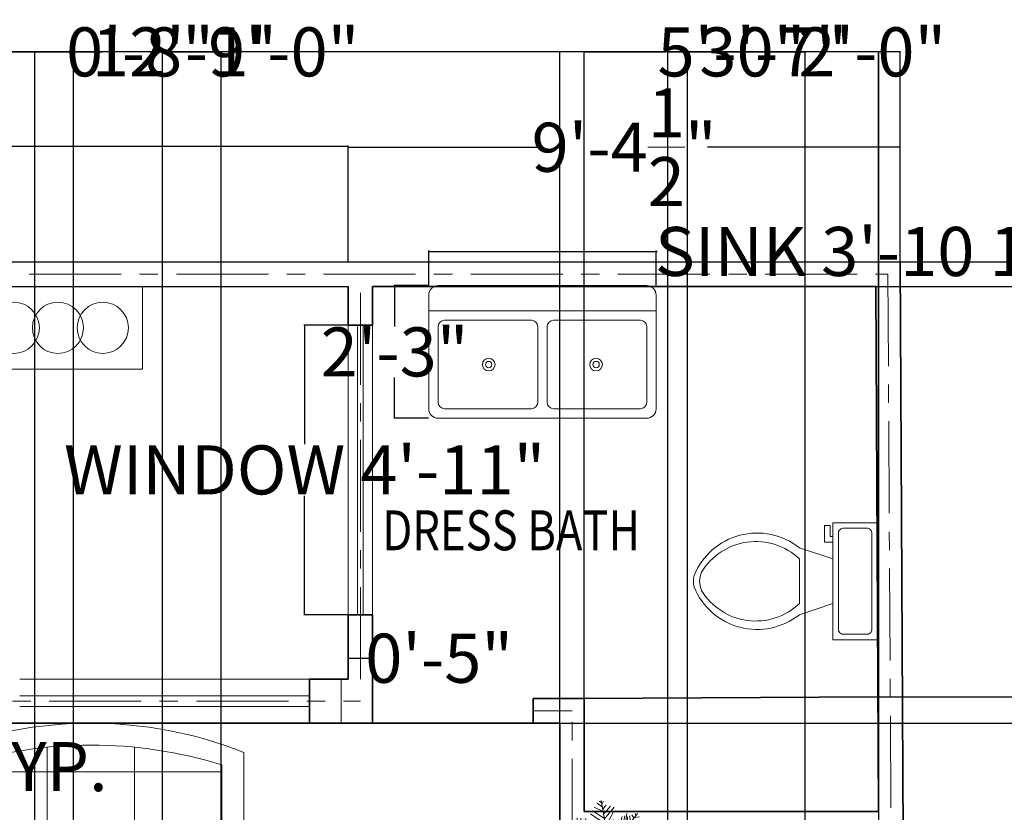
# Model space of a CAD drawing. Units: inches. Extents: x 541 to 1172, y -20 to 887.
# Tile 7 of 8: x 857 to 1058, y 717 to 879. Entities that reach past the tile are written whole.
import ezdxf

# ---------------------------------------------------------------- set-up
doc = ezdxf.new("R2010")
doc.units = ezdxf.units.IN
doc.header["$MEASUREMENT"] = 0
doc.linetypes.add('CENTER', pattern=[50.8, 31.75, -6.35, 6.35, -6.35])
doc.layers.get('0').update_dxf_attribs({"color": 70})
for name, color, linetype, lineweight in [('A-ANNO-DIMS', 2, 'Continuous', 18), ('A-AREA-IDEN', 7, 'Continuous', 20), ('A-FLOR-FIXT', 9, 'Continuous', 18), ('A-FURN', 30, 'Continuous', 18), ('A-WALL-CNTR', 1, 'CENTER', 13), ('C-PROP', 7, 'Continuous', 25), ('L-PLNT', 70, 'Continuous', 18), ('L-SITE-WALL', 7, 'Continuous', 30), ('WALL', 7, 'Continuous', 35), ('WINDOW', 2, 'Continuous', 18)]:
    doc.layers.add(name, color=color, linetype=linetype, lineweight=lineweight)
doc.styles.get("Standard").update_dxf_attribs({"font": 'arial.ttf'})
doc.styles.add('YQ_DIM', font='SUPEROS.SHX', dxfattribs={"width": 0.8, "bigfont": 'HZDX.SHX'})
doc.dimstyles.get("Standard").update_dxf_attribs({"dimtxt": 10, "dimasz": 0.18, "dimexe": 0.18, "dimexo": 0.0625, "dimgap": 0.09, "dimtad": 0, "dimtih": 1, "dimtoh": 1, "dimdec": 1, "dimzin": 0, "dimdsep": 46, "dimlunit": 4, "dimtxsty": 'Standard', "dimcen": 0.09, "dimadec": 0, "dimazin": 0, "dimtfac": 1, "dimtdec": 1, "dimtofl": 0, "dimtmove": 0, "dimatfit": 3, "dimfxl": 1, "dimtolj": 1, "dimtzin": 0, "dimarcsym": 0})

# ---------------------------------------------------------------- blocks, each defined once
blk = doc.blocks.new('*D1')
at = {"layer": 'A-ANNO-DIMS', "color": 0, "lineweight": -2, "transparency": 16777216}
for p, q in [((616.64, 829.74), (616.64, 853.38)), ((616.82, 853.2), (749.39, 853.2)), ((923.96, 853.2), (791.38, 853.2)), ((924.14, 829.74), (924.14, 853.38))]:
    blk.add_line(p, q, dxfattribs=at)
for points in [[(616.82, 853.23), (616.82, 853.17), (616.64, 853.2)], [(923.96, 853.23), (923.96, 853.17), (924.14, 853.2)]]:
    blk.add_solid(points, dxfattribs=at)
at = {"layer": 'Defpoints', "color": 0, "lineweight": -2, "transparency": 16777216}
for p in [(616.64, 853.2), (616.64, 829.68), (924.14, 829.68)]:
    blk.add_point(p, dxfattribs=at)
at = {"layer": 'A-ANNO-DIMS', "color": 0, "transparency": 16777216, "insert": (770.39, 853.2), "char_height": 10, "attachment_point": 5}
blk.add_mtext('\\A1;25\'-7{\\H1x;\\S1/2;}"', dxfattribs=at)
blk = doc.blocks.new('*D2')
at = {"layer": 'A-ANNO-DIMS', "color": 0, "lineweight": -2, "transparency": 16777216}
for p, q in [((924.14, 829.74), (924.14, 853.22)), ((924.32, 853.04), (963.36, 853.04)), ((1036.46, 853.04), (997.41, 853.04)), ((1036.64, 829.74), (1036.64, 853.22))]:
    blk.add_line(p, q, dxfattribs=at)
for points in [[(924.32, 853.07), (924.32, 853.01), (924.14, 853.04)], [(1036.46, 853.07), (1036.46, 853.01), (1036.64, 853.04)]]:
    blk.add_solid(points, dxfattribs=at)
at = {"layer": 'Defpoints', "color": 0, "lineweight": -2, "transparency": 16777216}
for p in [(1036.64, 853.04), (924.14, 829.68), (1036.64, 829.68)]:
    blk.add_point(p, dxfattribs=at)
at = {"layer": 'A-ANNO-DIMS', "color": 0, "transparency": 16777216, "insert": (980.39, 853.04), "char_height": 10, "attachment_point": 5}
blk.add_mtext('\\A1;9\'-4{\\H1x;\\S1/2;}"', dxfattribs=at)
blk = doc.blocks.new('Sofa - Roundback 7 ft.')
for p, q in [((-12.00002, -32.4421), (-12.00003, -6.5971)), ((11.99997, -32.4421), (11.99998, -6.5971)), ((-36.000027, -34), (-36.000027, -11.4696)), ((-35.999844, -13.3819), (35.9998, -13.3819)), ((35.99998, -34), (35.99998, -11.4696)), ((-36.000027, -32.4421), (35.99998, -32.4421))]:
    blk.add_line(p, q)
for points in [[(-36.000027, -34), (-42.000027, -34), (-42.000027, -8)], [(41.99998, -8), (41.99998, -34), (35.99998, -34)]]:
    blk.add_lwpolyline(points)
for centre, radius, start, end in [((0, -114.25), 114.25, 68.43141, 111.5686), ((-0.00001, -127.1968), 121.1968, 72.72033, 107.2797)]:
    blk.add_arc(centre, radius, start, end)
blk = doc.blocks.new('*U7')
for p, q in [((-8.737, 47.138), (-17.069, 52.711)), ((-10.186, 53.64), (-13.084, 55.962)), ((0, 0), (-10.5, 57)), ((-9.099, 51.782), (-6.563, 55.962)), ((-7.65, 43.423), (-2.578, 49.46)), ((-5.839, 35.992), (4.667, 48.067)), ((-3.665, 19.273), (-27.574, 35.527)), ((-5.114, 28.097), (-24.676, 40.636)), ((-7.288, 39.707), (-21.778, 46.673)), ((-5.114, 27.632), (10.463, 46.673)), ((-2.941, 16.486), (8.652, 37.85)), ((22.055, 7.198), (27.489, 32.277)), ((27, 9), (48, 36)), ((27.127, 9.056), (31.112, 35.992)), ((35.096, 32.741), (37.27, 22.524)), ((38.719, 34.134), (41.979, 28.561)), ((44.153, 36.456), (45.239, 32.741)), ((-47.498, 19.737), (-55.83, 18.344)), ((-31.5, 4.5), (-52.5, 25.5)), ((-48.585, 21.131), (-49.309, 29.026)), ((-43.513, 28.561), (-42.427, 15.558)), ((-38.442, 26.239), (-34.819, 7.663)), ((-35.544, 28.097), (-24.314, 3.947)), ((-14.533, 2.09), (-30.834, 25.31)), ((-24.314, 23.917), (-2.941, 13.7)), ((-1.129, 6.734), (9.014, 26.704)), ((3.942, 1.625), (11.187, 24.381)), ((10.101, 3.483), (17.708, 26.239)), ((16.259, 5.805), (23.142, 31.348)), ((31.836, 30.883), (32.561, 16.486)), ((33.285, 16.486), (48.862, 10.913)), ((36.183, 19.737), (48.137, 17.88)), ((40.53, 25.775), (48.862, 24.846)), ((43.791, 29.954), (51.036, 30.883)), ((-40.615, 13.7), (-55.105, 10.913)), ((-33.37, 6.269), (-52.207, 5.34)), ((-28.299, 3.483), (-47.86, -5.805)), ((-21.416, 3.018), (-38.079, -8.128)), ((0, 0), (-31.5, 4.5)), ((-15.982, 2.09), (-30.11, -9.521)), ((0, 0), (-22.5, -19.5)), ((-6.563, 1.161), (-21.416, -8.128)), ((-20.691, 13.7), (-1.129, 4.876)), ((0, 0), (27, 9)), ((0, 0), (18, -22.5)), ((6.478, 1.625), (26.04, -8.592)), ((11.187, 3.483), (30.749, -5.805)), ((18.07, 5.805), (35.096, -3.483)), ((24.229, 7.663), (46.688, 1.625)), ((29.662, 12.307), (48.137, 6.269)), ((-17.431, -15.094), (-42.789, -18.809)), ((-15.257, -12.772), (-30.11, -12.772)), ((-6.563, -5.805), (-19.967, -9.985)), ((-17.069, -15.094), (-12.721, -40.172)), ((-13.446, -11.378), (-8.737, -32.741)), ((-9.461, -8.592), (-6.201, -23.453)), ((-4.752, -3.483), (-3.665, -14.629)), ((2.493, -3.019), (-1.491, -20.202)), ((1.769, -2.555), (24.229, -9.521)), ((5.029, -6.27), (2.131, -25.775)), ((9.014, -11.378), (3.58, -35.992)), ((7.565, -9.056), (32.198, -14.629)), ((12.274, -15.094), (36.907, -18.809)), ((-28.299, -29.026), (-42.789, -31.348)), ((-24.314, -21.596), (-42.427, -22.06)), ((-26.849, -26.24), (-40.253, -25.775)), ((-22.5, -19.5), (-37.5, -45)), ((-29.023, -30.884), (-27.936, -43.887)), ((-25.038, -23.918), (-22.865, -45.281)), ((-20.691, -18.345), (-17.793, -44.352)), ((14.085, -16.951), (6.478, -40.172)), ((18.07, -22.524), (8.289, -45.745)), ((20.244, -30.419), (15.897, -44.816)), ((16.259, -19.738), (36.183, -22.989)), ((18, -22.5), (27, -52.5)), ((18.433, -22.524), (40.53, -29.026)), ((19.157, -25.311), (38.719, -33.206)), ((-30.834, -34.135), (-42.427, -35.528)), ((-34.457, -39.708), (-40.978, -42.494)), ((-32.646, -36.921), (-31.921, -44.352)), ((22.78, -37.85), (19.519, -48.532)), ((21.331, -32.741), (39.081, -40.636)), ((22.78, -38.314), (34.372, -44.816)), ((24.591, -45.745), (23.142, -50.854)), ((24.591, -43.423), (30.749, -47.603)), ((26.764, -49.925), (28.213, -50.854))]:
    blk.add_line(p, q)
blk = doc.blocks.new('WD_WIN4')
at = {"lineweight": -2}
for p, q in [((-0.5, 0.5), (0.5, 0.5)), ((-0.5, 0.12), (0.5, 0.12)), ((-0.5, -0.12), (0.5, -0.12)), ((-0.5, -0.5), (0.5, -0.5))]:
    blk.add_line(p, q, dxfattribs=at)
blk = doc.blocks.new('*U28')
for p, q in [((9.5, -6), (9.5, -2)), ((-10, -8.5), (-8, -8.5)), ((-10, -9.5), (-10, -8.5)), ((-8, -8.5), (-8, -8)), ((-7, -8), (-7, -9.5)), ((-4, -8), (-6, -14)), ((4, -8), (6, -14)), ((-7, -9.5), (-10, -9.5)), ((4, -14), (-4, -14))]:
    blk.add_line(p, q)
blk.add_lwpolyline([(10.5, -8), (10.5, 0), (-10.5, 0), (-10.5, -8)], close=True)
for points in [[(8.5, -1), (-8.5, -1)], [(-9.5, -2), (-9.5, -6)], [(-8.5, -7), (8.5, -7)]]:
    blk.add_lwpolyline(points)
for centre, radius, start, end in [((-8.62, -1.88), 0.884, 81.8699, 188.1301), ((8.62, -1.88), 0.884, 351.8699, 98.1301), ((-8.62, -6.12), 0.884, 171.8699, 278.1301), ((8.62, -6.12), 0.884, 261.8699, 8.1301), ((3.52, -21.58), 12.17, 141.4691, 247.9714), ((4.2, -21.82), 11.33, 136.3677, 238.9468), ((-3.52, -21.58), 12.17, 292.0284, 38.5307), ((-4.2, -21.82), 11.33, 301.053, 43.6321), ((0, -27.88), 4, 245.7318, 294.2682), ((0, -29), 4, 254.8605, 285.1395)]:
    blk.add_arc(centre, radius, start, end)
blk = doc.blocks.new('Sink-double - 36 in top')
for p, q in [((-18, -4), (18, -4)), ((-0.75, -18.5), (-0.75, -6.5)), ((0.75, -6.5), (0.75, -18.5))]:
    blk.add_line(p, q)
for points in [[(-16.5, 0), (16.5, 0)], [(-18, -19.5), (-18, -1.5)], [(18, -1.5), (18, -19.5)], [(-15.5, -5.5), (-1.75, -5.5)], [(1.75, -5.5), (15.5, -5.5)], [(-16.5, -18.5), (-16.5, -6.5)], [(16.5, -6.5), (16.5, -18.5)], [(-1.75, -19.5), (-15.5, -19.5)], [(15.5, -19.5), (1.75, -19.5)], [(16.5, -21), (-16.5, -21)]]:
    blk.add_lwpolyline(points)
for centre, radius in [((-8.5, -12.5), 1), ((-8.5, -12.5), 0.5), ((8.5, -12.5), 1), ((8.5, -12.5), 0.5)]:
    blk.add_circle(centre, radius)
for centre, radius, start, end in [((-16.5, -1.5), 1.5, 90, 180), ((16.5, -1.5), 1.5, 0, 90), ((-15.5, -6.5), 1, 90, 180), ((-1.75, -6.5), 1, 0, 90), ((1.75, -6.5), 1, 90, 180), ((15.5, -6.5), 1, 0, 90), ((-15.5, -18.5), 1, 180, 270), ((-1.75, -18.5), 1, 270, 0), ((1.75, -18.5), 1, 180, 270), ((15.5, -18.5), 1, 270, 0), ((-16.5, -19.5), 1.5, 180, 270), ((16.5, -19.5), 1.5, 270, 0)]:
    blk.add_arc(centre, radius, start, end)
blk = doc.blocks.new('PLANTER-THREE-ROUND')
blk.add_lwpolyline([(34.49, 16.89), (0, 16.89), (0, 0), (34.49, 0)], close=True)
for centre in [(8.25, 8.45), (17.25, 8.45), (26.39, 8.45)]:
    blk.add_circle(centre, 5.21)
blk = doc.blocks.new('*D39')
at = {"layer": 'A-ANNO-DIMS', "color": 0, "lineweight": -2, "transparency": 16777216}
for p, q in [((684.16, 735.59), (684.16, 726.62)), ((743.21, 735.59), (743.21, 726.62)), ((684.34, 726.8), (743.03, 726.8)), ((743.21, 726.8), (743.39, 726.8))]:
    blk.add_line(p, q, dxfattribs=at)
for points in [[(684.34, 726.83), (684.34, 726.77), (684.16, 726.8)], [(743.03, 726.83), (743.03, 726.77), (743.21, 726.8)]]:
    blk.add_solid(points, dxfattribs=at)
at = {"layer": 'Defpoints', "color": 0, "lineweight": -2, "transparency": 16777216}
for p in [(684.16, 735.65), (743.21, 735.65), (743.21, 726.8)]:
    blk.add_point(p, dxfattribs=at)
at = {"layer": 'A-ANNO-DIMS', "color": 0, "transparency": 16777216, "insert": (810.64, 726.8), "char_height": 10, "attachment_point": 5}
blk.add_mtext('\\A1;WINDOW 4\'-11" TYP.', dxfattribs=at)
blk = doc.blocks.new('*D41')
at = {"layer": 'A-ANNO-DIMS', "color": 0, "lineweight": -2, "transparency": 16777216}
for p, q in [((924.07, 816.81), (915.1, 816.81)), ((915.28, 816.63), (915.28, 792.54)), ((915.28, 757.93), (915.28, 782.01)), ((924.07, 757.75), (915.1, 757.75))]:
    blk.add_line(p, q, dxfattribs=at)
for points in [[(915.25, 816.63), (915.31, 816.63), (915.28, 816.81)], [(915.25, 757.93), (915.31, 757.93), (915.28, 757.75)]]:
    blk.add_solid(points, dxfattribs=at)
at = {"layer": 'Defpoints', "color": 0, "lineweight": -2, "transparency": 16777216}
for p in [(924.14, 816.81), (915.28, 757.75), (924.14, 757.75)]:
    blk.add_point(p, dxfattribs=at)
at = {"layer": 'A-ANNO-DIMS', "color": 0, "transparency": 16777216, "insert": (915.28, 787.28), "char_height": 10, "attachment_point": 5}
blk.add_mtext('\\A1;WINDOW 4\'-11"', dxfattribs=at)
blk = doc.blocks.new('*D42')
at = {"layer": 'A-ANNO-DIMS', "color": 0, "lineweight": -2, "transparency": 16777216}
for p, q in [((924.14, 757.69), (924.14, 748.71)), ((929.14, 757.69), (929.14, 748.71)), ((924.32, 748.89), (928.96, 748.89)), ((929.14, 748.89), (929.32, 748.89))]:
    blk.add_line(p, q, dxfattribs=at)
for points in [[(924.32, 748.92), (924.32, 748.86), (924.14, 748.89)], [(928.96, 748.92), (928.96, 748.86), (929.14, 748.89)]]:
    blk.add_solid(points, dxfattribs=at)
at = {"layer": 'Defpoints', "color": 0, "lineweight": -2, "transparency": 16777216}
for p in [(924.14, 757.75), (929.14, 757.75), (929.14, 748.89)]:
    blk.add_point(p, dxfattribs=at)
at = {"layer": 'A-ANNO-DIMS', "color": 0, "transparency": 16777216, "insert": (942.7, 748.89), "char_height": 10, "attachment_point": 5}
blk.add_mtext('\\A1;0\'-5"', dxfattribs=at)
blk = doc.blocks.new('*D53')
at = {"layer": 'A-ANNO-DIMS', "color": 0, "lineweight": -2, "transparency": 16777216}
for p, q in [((940.56, 824.91), (940.56, 831.98)), ((940.74, 831.8), (986.74, 831.8)), ((986.92, 824.91), (986.92, 831.98)), ((986.92, 831.8), (987.1, 831.8))]:
    blk.add_line(p, q, dxfattribs=at)
for points in [[(940.74, 831.83), (940.74, 831.77), (940.56, 831.8)], [(986.74, 831.83), (986.74, 831.77), (986.92, 831.8)]]:
    blk.add_solid(points, dxfattribs=at)
at = {"layer": 'Defpoints', "color": 0, "lineweight": -2, "transparency": 16777216}
for p in [(986.92, 831.8), (940.56, 824.85), (986.92, 824.85)]:
    blk.add_point(p, dxfattribs=at)
at = {"layer": 'A-ANNO-DIMS', "color": 0, "transparency": 16777216, "insert": (1034.24, 831.8), "char_height": 10, "attachment_point": 5}
blk.add_mtext('\\A1;SINK 3\'-10 1/2"', dxfattribs=at)
blk = doc.blocks.new('*D54')
at = {"layer": 'A-ANNO-DIMS', "color": 0, "lineweight": -2, "transparency": 16777216}
for p, q in [((940.5, 824.85), (933.43, 824.85)), ((933.61, 824.67), (933.61, 816.53)), ((933.61, 797.99), (933.61, 806.13)), ((940.5, 797.81), (933.43, 797.81))]:
    blk.add_line(p, q, dxfattribs=at)
for points in [[(933.58, 824.67), (933.64, 824.67), (933.61, 824.85)], [(933.58, 797.99), (933.64, 797.99), (933.61, 797.81)]]:
    blk.add_solid(points, dxfattribs=at)
at = {"layer": 'Defpoints', "color": 0, "lineweight": -2, "transparency": 16777216}
for p in [(933.61, 824.85), (940.56, 824.85), (940.56, 797.81)]:
    blk.add_point(p, dxfattribs=at)
at = {"layer": 'A-ANNO-DIMS', "color": 0, "transparency": 16777216, "insert": (933.61, 811.33), "char_height": 10, "attachment_point": 5}
blk.add_mtext('\\A1;2\'-3"', dxfattribs=at)
blk = doc.blocks.new('*D69')
at = {"layer": 'A-ANNO-DIMS', "color": 0, "lineweight": -2, "transparency": 16777216}
for p, q in [((616.64, 829.74), (616.64, 872.66)), ((616.82, 872.48), (809.37, 872.48)), ((1036.46, 872.48), (843.9, 872.48)), ((1036.64, 829.74), (1036.64, 872.66))]:
    blk.add_line(p, q, dxfattribs=at)
for points in [[(616.82, 872.51), (616.82, 872.45), (616.64, 872.48)], [(1036.46, 872.51), (1036.46, 872.45), (1036.64, 872.48)]]:
    blk.add_solid(points, dxfattribs=at)
at = {"layer": 'Defpoints', "color": 0, "lineweight": -2, "transparency": 16777216}
for p in [(1036.64, 872.48), (616.64, 829.68), (1036.64, 829.68)]:
    blk.add_point(p, dxfattribs=at)
at = {"layer": 'A-ANNO-DIMS', "color": 0, "transparency": 16777216, "insert": (826.64, 872.48), "char_height": 10, "attachment_point": 5}
blk.add_mtext('\\A1;35\'-0"', dxfattribs=at)
blk = doc.blocks.new('*D70')
at = {"layer": 'A-ANNO-DIMS', "color": 0, "lineweight": -2, "transparency": 16777216}
for p, q in [((1036.7, 829.68), (1143.21, 829.68)), ((1143.03, 829.5), (1143.03, 444.36)), ((1143.03, 48.83), (1143.03, 433.97)), ((1037.35, 48.65), (1143.21, 48.65))]:
    blk.add_line(p, q, dxfattribs=at)
for points in [[(1143, 829.5), (1143.06, 829.5), (1143.03, 829.68)], [(1143, 48.83), (1143.06, 48.83), (1143.03, 48.65)]]:
    blk.add_solid(points, dxfattribs=at)
at = {"layer": 'Defpoints', "color": 0, "lineweight": -2, "transparency": 16777216}
for p in [(1036.64, 829.68), (1037.28, 48.65), (1143.03, 48.65)]:
    blk.add_point(p, dxfattribs=at)
at = {"layer": 'A-ANNO-DIMS', "color": 0, "transparency": 16777216, "insert": (1143.03, 439.17), "char_height": 10, "attachment_point": 5}
blk.add_mtext('\\A1;65\'-1"', dxfattribs=at)
blk = doc.blocks.new('*D76')
at = {"layer": 'A-ANNO-DIMS', "color": 0, "lineweight": -2, "transparency": 16777216}
for p, q in [((814.28, 735.72), (814.28, 872.66)), ((814.46, 872.48), (873.99, 872.48)), ((967.1, 872.48), (907.58, 872.48)), ((967.28, 735.72), (967.28, 872.66))]:
    blk.add_line(p, q, dxfattribs=at)
for points in [[(814.46, 872.51), (814.46, 872.45), (814.28, 872.48)], [(967.1, 872.51), (967.1, 872.45), (967.28, 872.48)]]:
    blk.add_solid(points, dxfattribs=at)
at = {"layer": 'Defpoints', "color": 0, "lineweight": -2, "transparency": 16777216}
for p in [(967.28, 872.48), (814.28, 735.65), (967.28, 735.65)]:
    blk.add_point(p, dxfattribs=at)
at = {"layer": 'A-ANNO-DIMS', "color": 0, "transparency": 16777216, "insert": (890.78, 872.48), "char_height": 10, "attachment_point": 5}
blk.add_mtext('\\A1;12\'-9"', dxfattribs=at)
blk = doc.blocks.new('*D77')
at = {"layer": 'A-ANNO-DIMS', "color": 0, "lineweight": -2, "transparency": 16777216}
for p, q in [((972.28, 717.72), (972.28, 872.66)), ((972.46, 872.48), (988.89, 872.48)), ((1032.08, 872.48), (1015.65, 872.48)), ((1032.26, 717.72), (1032.26, 872.66))]:
    blk.add_line(p, q, dxfattribs=at)
for points in [[(972.46, 872.51), (972.46, 872.45), (972.28, 872.48)], [(1032.08, 872.51), (1032.08, 872.45), (1032.26, 872.48)]]:
    blk.add_solid(points, dxfattribs=at)
at = {"layer": 'Defpoints', "color": 0, "lineweight": -2, "transparency": 16777216}
for p in [(1032.26, 872.48), (972.28, 717.65), (1032.26, 717.65)]:
    blk.add_point(p, dxfattribs=at)
at = {"layer": 'A-ANNO-DIMS', "color": 0, "transparency": 16777216, "insert": (1002.27, 872.48), "char_height": 10, "attachment_point": 5}
blk.add_mtext('\\A1;5\'-0"', dxfattribs=at)
blk = doc.blocks.new('*D79')
at = {"layer": 'A-ANNO-DIMS', "color": 0, "lineweight": -2, "transparency": 16777216}
for p, q in [((1031.73, 824.68), (1143.21, 824.68)), ((1143.03, 824.5), (1143.03, 788.09)), ((1143.03, 741.17), (1143.03, 777.57)), ((1032.19, 740.99), (1143.21, 740.99))]:
    blk.add_line(p, q, dxfattribs=at)
for points in [[(1143, 824.5), (1143.06, 824.5), (1143.03, 824.68)], [(1143, 741.17), (1143.06, 741.17), (1143.03, 740.99)]]:
    blk.add_solid(points, dxfattribs=at)
at = {"layer": 'Defpoints', "color": 0, "lineweight": -2, "transparency": 16777216}
for p in [(1031.66, 824.68), (1032.13, 740.99), (1143.03, 740.99)]:
    blk.add_point(p, dxfattribs=at)
at = {"layer": 'A-ANNO-DIMS', "color": 0, "transparency": 16777216, "insert": (1143.03, 782.83), "char_height": 10, "attachment_point": 5}
blk.add_mtext('\\A1;6\'-11 1/2"', dxfattribs=at)
blk = doc.blocks.new('*D89')
at = {"layer": 'A-ANNO-DIMS', "color": 0, "lineweight": -2, "transparency": 16777216}
for p, q in [((989.28, 430.72), (989.28, 872.66)), ((989.46, 872.48), (997.41, 872.48)), ((1032.1, 872.48), (1024.16, 872.48)), ((1032.28, 430.72), (1032.28, 872.66))]:
    blk.add_line(p, q, dxfattribs=at)
for points in [[(989.46, 872.51), (989.46, 872.45), (989.28, 872.48)], [(1032.1, 872.51), (1032.1, 872.45), (1032.28, 872.48)]]:
    blk.add_solid(points, dxfattribs=at)
at = {"layer": 'Defpoints', "color": 0, "lineweight": -2, "transparency": 16777216}
for p in [(1032.28, 872.48), (989.28, 430.65), (1032.28, 430.65)]:
    blk.add_point(p, dxfattribs=at)
at = {"layer": 'A-ANNO-DIMS', "color": 0, "transparency": 16777216, "insert": (1010.78, 872.48), "char_height": 10, "attachment_point": 5}
blk.add_mtext('\\A1;3\'-7"', dxfattribs=at)
blk = doc.blocks.new('*D97')
at = {"layer": 'A-ANNO-DIMS', "color": 0, "lineweight": -2, "transparency": 16777216}
for p, q in [((886.28, 430.72), (886.28, 872.66)), ((886.46, 872.48), (898.1, 872.48)), ((898.28, 430.72), (898.28, 872.66)), ((898.28, 872.48), (898.46, 872.48))]:
    blk.add_line(p, q, dxfattribs=at)
for points in [[(886.46, 872.51), (886.46, 872.45), (886.28, 872.48)], [(898.1, 872.51), (898.1, 872.45), (898.28, 872.48)]]:
    blk.add_solid(points, dxfattribs=at)
at = {"layer": 'Defpoints', "color": 0, "lineweight": -2, "transparency": 16777216}
for p in [(898.28, 872.48), (886.28, 430.65), (898.28, 430.65)]:
    blk.add_point(p, dxfattribs=at)
at = {"layer": 'A-ANNO-DIMS', "color": 0, "transparency": 16777216, "insert": (911.37, 872.48), "char_height": 10, "attachment_point": 5}
blk.add_mtext('\\A1;1\'-0"', dxfattribs=at)
blk = doc.blocks.new('*D98')
at = {"layer": 'A-ANNO-DIMS', "color": 0, "lineweight": -2, "transparency": 16777216}
for p, q in [((993.28, 326.72), (993.28, 872.66)), ((993.46, 872.48), (1017.14, 872.48)), ((1017.32, 326.72), (1017.32, 872.66)), ((1017.32, 872.48), (1017.5, 872.48))]:
    blk.add_line(p, q, dxfattribs=at)
for points in [[(993.46, 872.51), (993.46, 872.45), (993.28, 872.48)], [(1017.14, 872.51), (1017.14, 872.45), (1017.32, 872.48)]]:
    blk.add_solid(points, dxfattribs=at)
at = {"layer": 'Defpoints', "color": 0, "lineweight": -2, "transparency": 16777216}
for p in [(1017.32, 872.48), (993.28, 326.65), (1017.32, 326.65)]:
    blk.add_point(p, dxfattribs=at)
at = {"layer": 'A-ANNO-DIMS', "color": 0, "transparency": 16777216, "insert": (1030.97, 872.48), "char_height": 10, "attachment_point": 5}
blk.add_mtext('\\A1;2\'-0"', dxfattribs=at)
blk = doc.blocks.new('*D101')
at = {"layer": 'A-ANNO-DIMS', "color": 0, "lineweight": -2, "transparency": 16777216}
for p, q in [((805.35, 735.65), (1143.21, 735.65)), ((1143.03, 735.47), (1143.03, 730.35)), ((1143.03, 714.83), (1143.03, 719.96)), ((805.35, 714.65), (1143.21, 714.65))]:
    blk.add_line(p, q, dxfattribs=at)
for points in [[(1143, 735.47), (1143.06, 735.47), (1143.03, 735.65)], [(1143, 714.83), (1143.06, 714.83), (1143.03, 714.65)]]:
    blk.add_solid(points, dxfattribs=at)
at = {"layer": 'Defpoints', "color": 0, "lineweight": -2, "transparency": 16777216}
for p in [(805.28, 735.65), (1143.03, 735.65), (805.28, 714.65)]:
    blk.add_point(p, dxfattribs=at)
at = {"layer": 'A-ANNO-DIMS', "color": 0, "transparency": 16777216, "insert": (1143.03, 725.15), "char_height": 10, "attachment_point": 5}
blk.add_mtext('\\A1;1\'-9"', dxfattribs=at)
blk = doc.blocks.new('*D104')
at = {"layer": 'A-ANNO-DIMS', "color": 0, "lineweight": -2, "transparency": 16777216}
for p, q in [((860.28, 177.72), (860.28, 872.66)), ((860.46, 872.48), (867.98, 872.48)), ((868.16, 177.72), (868.16, 872.66)), ((868.16, 872.48), (868.34, 872.48))]:
    blk.add_line(p, q, dxfattribs=at)
for points in [[(860.46, 872.51), (860.46, 872.45), (860.28, 872.48)], [(867.98, 872.51), (867.98, 872.45), (868.16, 872.48)]]:
    blk.add_solid(points, dxfattribs=at)
at = {"layer": 'Defpoints', "color": 0, "lineweight": -2, "transparency": 16777216}
for p in [(868.16, 872.48), (860.28, 177.65), (868.16, 177.65)]:
    blk.add_point(p, dxfattribs=at)
at = {"layer": 'A-ANNO-DIMS', "color": 0, "transparency": 16777216, "insert": (881.72, 872.48), "char_height": 10, "attachment_point": 5}
blk.add_mtext('\\A1;0\'-8"', dxfattribs=at)
blk = doc.blocks.new('*D107')
at = {"layer": 'A-ANNO-DIMS', "color": 0, "lineweight": -2, "transparency": 16777216}
for p, q in [((967.22, 735.65), (573.66, 735.65)), ((573.84, 735.47), (573.84, 668.85)), ((573.84, 591.83), (573.84, 658.46)), ((967.22, 591.65), (573.66, 591.65))]:
    blk.add_line(p, q, dxfattribs=at)
for points in [[(573.81, 735.47), (573.87, 735.47), (573.84, 735.65)], [(573.81, 591.83), (573.87, 591.83), (573.84, 591.65)]]:
    blk.add_solid(points, dxfattribs=at)
at = {"layer": 'Defpoints', "color": 0, "lineweight": -2, "transparency": 16777216}
for p in [(967.28, 735.65), (573.84, 591.65), (967.28, 591.65)]:
    blk.add_point(p, dxfattribs=at)
at = {"layer": 'A-ANNO-DIMS', "color": 0, "transparency": 16777216, "insert": (573.84, 663.65), "char_height": 10, "attachment_point": 5}
blk.add_mtext('\\A1;12\'-0"', dxfattribs=at)

msp = doc.modelspace()

# ---------------------------------------------------------------- linework, layer by layer
at = {"layer": 'A-WALL-CNTR', "ltscale": 0.590551}
for p, q in [((619.14, 827.18), (1034.15, 827.18)), ((1034.15, 827.18), (1034.77, 715.15)), ((926.64, 744.65), (926.64, 824.68)), ((922.7, 735.65), (922.7, 744.65)), ((743.21, 740.15), (926.64, 740.15)), ((961.84, 738.15), (969.78, 738.15)), ((969.78, 589.65), (969.78, 738.15))]:
    msp.add_line(p, q, dxfattribs=at)
at = {"layer": 'C-PROP'}
msp.add_line((616.64, 829.68), (1036.64, 829.68), dxfattribs=at)
at = {"layer": 'L-SITE-WALL'}
for p, q in [((616.64, 829.68), (1036.64, 829.68)), ((621.64, 824.68), (924.14, 824.68))]:
    msp.add_line(p, q, dxfattribs=at)
at = {"layer": 'WALL'}
for p, q in [((1036.64, 829.68), (1037.28, 712.65)), ((924.14, 816.81), (924.14, 824.68)), ((929.14, 824.68), (1031.66, 824.68)), ((929.14, 816.81), (929.14, 824.68)), ((1031.66, 824.68), (1032.26, 717.65)), ((924.14, 816.81), (929.14, 816.81)), ((924.14, 744.65), (924.14, 757.75)), ((924.14, 757.75), (929.14, 757.75)), ((929.14, 735.65), (929.14, 757.75)), ((916.26, 744.65), (924.14, 744.65)), ((916.26, 744.65), (916.26, 735.65)), ((972.28, 740.65), (961.84, 740.65)), ((961.84, 740.65), (961.84, 735.65)), ((972.28, 740.65), (1032.13, 740.99)), ((972.28, 735.65), (972.28, 740.65)), ((916.26, 735.65), (929.14, 735.65)), ((961.84, 735.65), (967.28, 735.65)), ((967.28, 735.65), (967.28, 712.65)), ((972.28, 717.65), (972.28, 735.65)), ((972.28, 717.65), (1032.26, 717.65))]:
    msp.add_line(p, q, dxfattribs=at)

# ---------------------------------------------------------------- block references
at = {"layer": 'A-FLOR-FIXT', "xscale": 1.287660258812461, "yscale": 1.287660258812461, "zscale": 1.287660258812461}
msp.add_blockref('Sink-double - 36 in top', (963.74, 824.85), dxfattribs=at)
at = {"layer": 'A-FLOR-FIXT', "xscale": 1.136782620355255, "yscale": 1.136782620355255, "zscale": 1.136782620355255, "rotation": 270.0000000000004}
msp.add_blockref('*U28', (1032.02, 764.58), dxfattribs=at)
at = {"layer": 'A-FURN', "xscale": 0.7424226432878923, "yscale": 0.7424226432878923, "zscale": 0.7424226432878923}
msp.add_blockref('Sofa - Roundback 7 ft.', (871.71, 735.65), dxfattribs=at)
at = {"layer": 'L-PLNT'}
msp.add_blockref('PLANTER-THREE-ROUND', (847.75, 807.79), dxfattribs=at)
at = {"layer": 'L-PLNT', "xscale": 0.1264207715891114, "yscale": 0.1264207715891114, "zscale": 0.1264207715891114}
msp.add_blockref('*U7', (977.04, 712.66), dxfattribs=at)
at = {"layer": 'WINDOW', "xscale": 59.05511811023622, "zscale": 59.05511811023622}
for p, yscale, rotation in [((926.64, 787.28), 5.000000000002842, 270.0000000000009), ((886.73, 740.15), 9, 179.9999999999998)]:
    msp.add_blockref('WD_WIN4', p, dxfattribs=dict(at, yscale=yscale, rotation=rotation))

# ---------------------------------------------------------------- texts
at = {"layer": 'A-AREA-IDEN', "style": 'YQ_DIM', "width": 0.8}
msp.add_text(' DRESS BATH', height=8.1299, dxfattribs=at).set_placement((929.14, 770.9))

# ---------------------------------------------------------------- dimensions: what is measured, and where the dimension line sits
at = {"layer": 'A-ANNO-DIMS'}
for base, p1, p2, override, picture, middle in [((1036.64, 872.48), (616.64, 829.68), (1036.64, 829.68), {"dimdec": 1, "dimlfac": 1, "dimrnd": 0, "dimzin": 1, "dimdsep": 46, "dimlunit": 4, "dimfrac": 2}, '*D69', (826.64, 872.48)), ((967.28, 872.48), (814.28, 735.65), (967.28, 735.65), {"dimdec": 1, "dimlfac": 1, "dimrnd": 0, "dimzin": 1, "dimdsep": 46, "dimlunit": 4, "dimfrac": 2}, '*D76', (890.78, 872.48)), ((868.16, 872.48), (860.28, 177.65), (868.16, 177.65), {"dimdec": 1, "dimlfac": 1, "dimrnd": 0, "dimzin": 1, "dimdsep": 46, "dimlunit": 4, "dimfrac": 2}, '*D104', (881.72, 872.48)), ((898.28, 872.48), (886.28, 430.65), (898.28, 430.65), {"dimdec": 1, "dimlfac": 1, "dimrnd": 0, "dimzin": 1, "dimdsep": 46, "dimlunit": 4, "dimfrac": 2}, '*D97', (911.37, 872.48)), ((1032.26, 872.48), (972.28, 717.65), (1032.26, 717.65), {"dimdec": 1, "dimlfac": 1, "dimrnd": 0, "dimzin": 1, "dimdsep": 46, "dimlunit": 4, "dimfrac": 2}, '*D77', (1002.27, 872.48)), ((1032.28, 872.48), (989.28, 430.65), (1032.28, 430.65), {"dimdec": 1, "dimlfac": 1, "dimrnd": 0, "dimzin": 1, "dimdsep": 46, "dimlunit": 4, "dimfrac": 2}, '*D89', (1010.78, 872.48)), ((1017.32, 872.48), (993.28, 326.65), (1017.32, 326.65), {"dimdec": 1, "dimlfac": 1, "dimrnd": 0, "dimzin": 1, "dimdsep": 46, "dimlunit": 4, "dimfrac": 2}, '*D98', (1030.97, 872.48)), ((616.64, 853.2), (924.14, 829.68), (616.64, 829.68), {"dimclrd": 0, "dimclre": 0, "dimclrt": 0}, '*D1', (770.39, 853.2)), ((1036.64, 853.04), (924.14, 829.68), (1036.64, 829.68), {"dimclrd": 0, "dimclre": 0, "dimclrt": 0}, '*D2', (980.39, 853.04)), ((929.14, 748.89), (924.14, 757.75), (929.14, 757.75), {"dimdec": 1, "dimlfac": 1, "dimrnd": 0, "dimzin": 1, "dimdsep": 46, "dimlunit": 4, "dimfrac": 2}, '*D42', (942.7, 748.89))]:
    dim = msp.add_linear_dim(base=base, p1=p1, p2=p2, dimstyle='Standard', override=override, dxfattribs=at)
    dim.commit()
    dim.dimension.update_dxf_attribs({"geometry": picture, "text_midpoint": middle})
for base, p1, p2, text, picture, middle in [((986.92, 831.8), (940.56, 824.85), (986.92, 824.85), 'SINK <>', '*D53', (1034.24, 831.8)), ((743.2125, 726.7962), (684.1574, 735.6544), (743.2125, 735.6544), 'WINDOW <> TYP.', '*D39', (810.638, 726.7962))]:
    dim = msp.add_linear_dim(base=base, p1=p1, p2=p2, text=text, dimstyle='Standard', override={"dimdec": 1, "dimlfac": 1, "dimrnd": 0, "dimzin": 1, "dimdsep": 46, "dimlunit": 4, "dimfrac": 2}, dxfattribs=at)
    dim.commit()
    dim.dimension.update_dxf_attribs({"geometry": picture, "text_midpoint": middle})
for base, p1, p2, picture, middle in [((1143.03, 48.65), (1036.64, 829.68), (1037.28, 48.65), '*D70', (1143.03, 439.17)), ((933.61, 824.85), (940.56, 797.81), (940.56, 824.85), '*D54', (933.61, 811.33)), ((1143.03, 740.99), (1031.66, 824.68), (1032.13, 740.99), '*D79', (1143.03, 782.83)), ((573.84, 591.65), (967.28, 735.65), (967.28, 591.65), '*D107', (573.84, 663.65)), ((1143.03, 735.65), (805.28, 714.65), (805.28, 735.65), '*D101', (1143.03, 725.15))]:
    dim = msp.add_linear_dim(base=base, p1=p1, p2=p2, angle=90, dimstyle='Standard', override={"dimdec": 1, "dimlfac": 1, "dimrnd": 0, "dimzin": 1, "dimdsep": 46, "dimlunit": 4, "dimfrac": 2}, dxfattribs=at)
    dim.commit()
    dim.dimension.update_dxf_attribs({"geometry": picture, "text_midpoint": middle})
dim = msp.add_linear_dim(base=(915.28, 757.75), p1=(924.14, 816.81), p2=(924.14, 757.75), angle=270, text='WINDOW <>', dimstyle='Standard', override={"dimdec": 1, "dimlfac": 1, "dimrnd": 0, "dimzin": 1, "dimdsep": 46, "dimlunit": 4, "dimfrac": 2}, dxfattribs=at)
dim.commit()
dim.dimension.update_dxf_attribs({"geometry": '*D41', "text_midpoint": (915.28, 787.28)})

doc.saveas('drawing.dxf')
